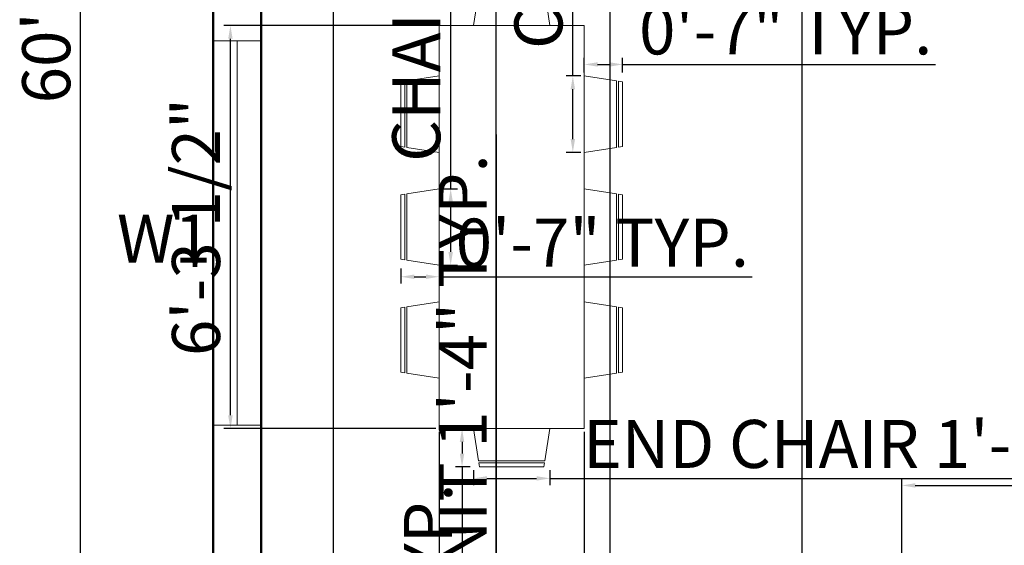
# Model space of a CAD drawing. Units: inches. Extents: x 3587 to 4539, y 1613 to 2440.
# Tile 3 of 8: x 3608 to 3793, y 1928 to 2027. Entities that reach past the tile are written whole.
import ezdxf

# ---------------------------------------------------------------- set-up
doc = ezdxf.new("R2010")
doc.units = ezdxf.units.IN
for name, color, linetype, lineweight in [('A-ANNO-DIMS', 2, 'Continuous', 18), ('A-ANNO-TEXT', 7, 'Continuous', 18), ('A-FURN', 8, 'Continuous', 18), ('A-GLAZ', 4, 'Continuous', 20), ('A-WALL', 7, 'Continuous', 50)]:
    doc.layers.add(name, color=color, linetype=linetype, lineweight=lineweight)
doc.styles.get("Standard").update_dxf_attribs({"font": 'arial.ttf'})
doc.dimstyles.new('ISO-25', dxfattribs={"dimtxt": 9, "dimasz": 2.5, "dimexe": 1.25, "dimexo": 0.625, "dimtad": 1, "dimlunit": 3, "dimtxsty": 'Standard', "dimcen": 2.5, "dimadec": 0, "dimazin": 0, "dimtfac": 1, "dimtmove": 0, "dimatfit": 3, "dimfxl": 1, "dimarcsym": 0})

# ---------------------------------------------------------------- blocks, each defined once
blk = doc.blocks.new('*D14')
at = {"layer": 'A-ANNO-DIMS', "color": 0, "lineweight": -2, "transparency": 16777216}
for p, q in [((3643.9, 2372.93), (3618.39, 2372.93)), ((3619.64, 2370.43), (3619.64, 1655.43)), ((3643.9, 1652.93), (3618.39, 1652.93))]:
    blk.add_line(p, q, dxfattribs=at)
at = {"layer": 'A-ANNO-DIMS', "color": 0, "transparency": 16777216}
for points in [[(3619.22, 2370.43), (3620.05, 2370.43), (3619.64, 2372.93)], [(3619.22, 1655.43), (3620.05, 1655.43), (3619.64, 1652.93)]]:
    blk.add_solid(points, dxfattribs=at)
at = {"layer": 'Defpoints', "color": 0, "transparency": 16777216}
for p in [(3644.52, 2372.93), (3619.64, 1652.93), (3644.52, 1652.93)]:
    blk.add_point(p, dxfattribs=at)
at = {"layer": 'A-ANNO-DIMS', "color": 0, "transparency": 16777216, "insert": (3614.42, 2019.45), "char_height": 9, "attachment_point": 5, "rotation": 90}
blk.add_mtext("60'", dxfattribs=at)
blk = doc.blocks.new('*D27')
at = {"layer": 'A-ANNO-DIMS', "color": 0, "lineweight": -2, "transparency": 16777216}
for p, q in [((3773.52, 1812.56), (3773.52, 1940.63)), ((3995.52, 1812.56), (3995.52, 1940.63)), ((3776.02, 1939.38), (3993.02, 1939.38))]:
    blk.add_line(p, q, dxfattribs=at)
at = {"layer": 'A-ANNO-DIMS', "color": 0, "transparency": 16777216}
for points in [[(3776.02, 1939.8), (3776.02, 1938.96), (3773.52, 1939.38)], [(3993.02, 1939.8), (3993.02, 1938.96), (3995.52, 1939.38)]]:
    blk.add_solid(points, dxfattribs=at)
at = {"layer": 'Defpoints', "color": 0, "transparency": 16777216}
for p in [(3995.52, 1939.38), (3773.52, 1811.93), (3995.52, 1811.93)]:
    blk.add_point(p, dxfattribs=at)
at = {"layer": 'A-ANNO-DIMS', "color": 0, "transparency": 16777216, "insert": (3884.52, 1944.6), "char_height": 9, "attachment_point": 5}
blk.add_mtext('18\'-6"', dxfattribs=at)
blk = doc.blocks.new('DINING-CHAIR-SIDE-R')
for p, q in [((6.04, 13.38), (0, 14.32)), ((6.04, 13.37), (6.04, 0.94)), ((7.17, 13.2), (6.42, 13.32)), ((6.42, 1), (6.42, 13.31)), ((7.17, 13.2), (7.17, 1.12)), ((0, 0), (6.04, 0.94)), ((6.42, 1), (7.17, 1.12))]:
    blk.add_line(p, q)
blk = doc.blocks.new('DINING-CHAIR-SIDE-L')
for p, q in [((0, 13.2), (0.75, 13.32)), ((0, 13.2), (0, 1.12)), ((0.75, 1), (0.75, 13.31)), ((1.13, 13.38), (7.17, 14.32)), ((1.13, 13.37), (1.13, 0.94)), ((0.75, 1), (0, 1.12)), ((7.17, 0), (1.13, 0.94))]:
    blk.add_line(p, q)
blk = doc.blocks.new('DINING-CHAIR-END')
for p, q in [((0, 0), (0.94, 6.04)), ((13.37, 6.04), (0.94, 6.04)), ((1, 6.42), (1.12, 7.17)), ((1, 6.42), (13.32, 6.42)), ((13.2, 7.17), (1.12, 7.17)), ((13.2, 7.17), (13.32, 6.42)), ((13.38, 6.04), (14.32, 0))]:
    blk.add_line(p, q)
blk = doc.blocks.new('*D70')
at = {"layer": 'A-ANNO-DIMS', "color": 0, "lineweight": -2, "transparency": 16777216}
for p, q in [((3697.61, 1857.46), (3697.61, 2005.08)), ((3695.87, 1857.46), (3698.86, 1857.46)), ((3697.61, 1844.2), (3697.61, 1854.96)), ((3695.87, 1841.7), (3698.86, 1841.7))]:
    blk.add_line(p, q, dxfattribs=at)
at = {"layer": 'A-ANNO-DIMS', "color": 0, "transparency": 16777216}
for points in [[(3697.19, 1854.96), (3698.02, 1854.96), (3697.61, 1857.46)], [(3697.19, 1844.2), (3698.02, 1844.2), (3697.61, 1841.7)]]:
    blk.add_solid(points, dxfattribs=at)
at = {"layer": 'Defpoints', "color": 0, "transparency": 16777216}
for p in [(3695.24, 1857.46), (3697.61, 1857.46), (3695.24, 1841.7)]:
    blk.add_point(p, dxfattribs=at)
at = {"layer": 'A-ANNO-DIMS', "color": 0, "transparency": 16777216, "insert": (3692.39, 1932.52), "char_height": 9, "attachment_point": 5, "rotation": 90}
blk.add_mtext('BURNER UNIT 1\'-4" TYP.', dxfattribs=at)
blk = doc.blocks.new('*D74')
at = {"layer": 'A-ANNO-DIMS', "color": 0, "lineweight": -2, "transparency": 16777216}
for p, q in [((3711.88, 2016.07), (3711.88, 2138.15)), ((3713.4, 2016.07), (3710.63, 2016.07)), ((3711.88, 2004.25), (3711.88, 2013.57)), ((3713.4, 2001.75), (3710.63, 2001.75))]:
    blk.add_line(p, q, dxfattribs=at)
at = {"layer": 'A-ANNO-DIMS', "color": 0, "transparency": 16777216}
for points in [[(3711.46, 2013.57), (3712.29, 2013.57), (3711.88, 2016.07)], [(3711.46, 2004.25), (3712.29, 2004.25), (3711.88, 2001.75)]]:
    blk.add_solid(points, dxfattribs=at)
at = {"layer": 'Defpoints', "color": 0, "transparency": 16777216}
for p in [(3711.88, 2016.07), (3714.02, 2016.07), (3714.02, 2001.75)]:
    blk.add_point(p, dxfattribs=at)
at = {"layer": 'A-ANNO-DIMS', "color": 0, "transparency": 16777216, "insert": (3706.6, 2078.36), "char_height": 9, "attachment_point": 5, "rotation": 90}
blk.add_mtext('CHAIR 1\'-2 1/2" TYP.', dxfattribs=at)
blk = doc.blocks.new('*D75')
at = {"layer": 'A-ANNO-DIMS', "color": 0, "lineweight": -2, "transparency": 16777216}
for p, q in [((3714.02, 2016.69), (3714.02, 2019.46)), ((3721.2, 2016.69), (3721.2, 2019.46)), ((3716.52, 2018.21), (3718.7, 2018.21)), ((3721.2, 2018.21), (3779.81, 2018.21))]:
    blk.add_line(p, q, dxfattribs=at)
at = {"layer": 'A-ANNO-DIMS', "color": 0, "transparency": 16777216}
for points in [[(3716.52, 2018.63), (3716.52, 2017.8), (3714.02, 2018.21)], [(3718.7, 2018.63), (3718.7, 2017.8), (3721.2, 2018.21)]]:
    blk.add_solid(points, dxfattribs=at)
at = {"layer": 'Defpoints', "color": 0, "transparency": 16777216}
for p in [(3721.2, 2018.21), (3714.02, 2016.07), (3721.2, 2016.07)]:
    blk.add_point(p, dxfattribs=at)
at = {"layer": 'A-ANNO-DIMS', "color": 0, "transparency": 16777216, "insert": (3751.75, 2023.43), "char_height": 9, "attachment_point": 5}
blk.add_mtext('0\'-7" TYP.', dxfattribs=at)
blk = doc.blocks.new('*D76')
at = {"layer": 'A-ANNO-DIMS', "color": 0, "lineweight": -2, "transparency": 16777216}
for p, q in [((3689, 1994.93), (3689, 2117.02)), ((3687.48, 1994.93), (3690.25, 1994.93)), ((3689, 1983.11), (3689, 1992.43)), ((3687.48, 1980.61), (3690.25, 1980.61))]:
    blk.add_line(p, q, dxfattribs=at)
at = {"layer": 'A-ANNO-DIMS', "color": 0, "transparency": 16777216}
for points in [[(3688.58, 1992.43), (3689.42, 1992.43), (3689, 1994.93)], [(3688.58, 1983.11), (3689.42, 1983.11), (3689, 1980.61)]]:
    blk.add_solid(points, dxfattribs=at)
at = {"layer": 'Defpoints', "color": 0, "transparency": 16777216}
for p in [(3686.85, 1994.93), (3689, 1994.93), (3686.85, 1980.61)]:
    blk.add_point(p, dxfattribs=at)
at = {"layer": 'A-ANNO-DIMS', "color": 0, "transparency": 16777216, "insert": (3683.72, 2057.22), "char_height": 9, "attachment_point": 5, "rotation": 90}
blk.add_mtext('CHAIR 1\'-2 1/2" TYP.', dxfattribs=at)
blk = doc.blocks.new('*D77')
at = {"layer": 'A-ANNO-DIMS', "color": 0, "lineweight": -2, "transparency": 16777216}
for p, q in [((3679.68, 1979.98), (3679.68, 1977.21)), ((3686.85, 1979.98), (3686.85, 1977.21)), ((3682.18, 1978.46), (3684.35, 1978.46)), ((3686.85, 1978.46), (3745.46, 1978.46))]:
    blk.add_line(p, q, dxfattribs=at)
at = {"layer": 'A-ANNO-DIMS', "color": 0, "transparency": 16777216}
for points in [[(3682.18, 1978.88), (3682.18, 1978.04), (3679.68, 1978.46)], [(3684.35, 1978.88), (3684.35, 1978.04), (3686.85, 1978.46)]]:
    blk.add_solid(points, dxfattribs=at)
at = {"layer": 'Defpoints', "color": 0, "transparency": 16777216}
for p in [(3679.68, 1980.61), (3686.85, 1980.61), (3686.85, 1978.46)]:
    blk.add_point(p, dxfattribs=at)
at = {"layer": 'A-ANNO-DIMS', "color": 0, "transparency": 16777216, "insert": (3717.41, 1983.68), "char_height": 9, "attachment_point": 5}
blk.add_mtext('0\'-7" TYP.', dxfattribs=at)
blk = doc.blocks.new('*D78')
at = {"layer": 'A-ANNO-DIMS', "color": 0, "lineweight": -2, "transparency": 16777216}
for p, q in [((3693.28, 1942.22), (3693.28, 1939.45)), ((3707.6, 1942.22), (3707.6, 1939.45)), ((3695.78, 1940.7), (3705.1, 1940.7)), ((3707.6, 1940.7), (3859.36, 1940.7))]:
    blk.add_line(p, q, dxfattribs=at)
at = {"layer": 'A-ANNO-DIMS', "color": 0, "transparency": 16777216}
for points in [[(3695.78, 1941.11), (3695.78, 1940.28), (3693.28, 1940.7)], [(3705.1, 1941.11), (3705.1, 1940.28), (3707.6, 1940.7)]]:
    blk.add_solid(points, dxfattribs=at)
at = {"layer": 'Defpoints', "color": 0, "transparency": 16777216}
for p in [(3693.28, 1942.85), (3707.6, 1942.85), (3707.6, 1940.7)]:
    blk.add_point(p, dxfattribs=at)
at = {"layer": 'A-ANNO-DIMS', "color": 0, "transparency": 16777216, "insert": (3784.73, 1945.98), "char_height": 9, "attachment_point": 5}
blk.add_mtext('END CHAIR 1\'-2 1/2" TYP.', dxfattribs=at)
blk = doc.blocks.new('*D79')
at = {"layer": 'A-ANNO-DIMS', "color": 0, "lineweight": -2, "transparency": 16777216}
for p, q in [((3692.65, 1950.02), (3689.88, 1950.02)), ((3691.13, 1947.52), (3691.13, 1945.35)), ((3692.65, 1942.85), (3689.88, 1942.85)), ((3691.13, 1942.85), (3691.13, 1884.24))]:
    blk.add_line(p, q, dxfattribs=at)
at = {"layer": 'A-ANNO-DIMS', "color": 0, "transparency": 16777216}
for points in [[(3690.71, 1947.52), (3691.55, 1947.52), (3691.13, 1950.02)], [(3690.71, 1945.35), (3691.55, 1945.35), (3691.13, 1942.85)]]:
    blk.add_solid(points, dxfattribs=at)
at = {"layer": 'Defpoints', "color": 0, "transparency": 16777216}
for p in [(3693.28, 1950.02), (3691.13, 1942.85), (3693.28, 1942.85)]:
    blk.add_point(p, dxfattribs=at)
at = {"layer": 'A-ANNO-DIMS', "color": 0, "transparency": 16777216, "insert": (3685.91, 1912.29), "char_height": 9, "attachment_point": 5, "rotation": 90}
blk.add_mtext('0\'-7" TYP.', dxfattribs=at)
blk = doc.blocks.new('*D84')
at = {"layer": 'A-ANNO-DIMS', "color": 0, "lineweight": -2, "transparency": 16777216}
for p, q in [((3686.23, 2025.51), (3646.5, 2025.51)), ((3647.75, 1952.52), (3647.75, 2023.01)), ((3686.23, 1950.02), (3646.5, 1950.02))]:
    blk.add_line(p, q, dxfattribs=at)
at = {"layer": 'A-ANNO-DIMS', "color": 0, "transparency": 16777216}
for points in [[(3647.33, 2023.01), (3648.17, 2023.01), (3647.75, 2025.51)], [(3647.33, 1952.52), (3648.17, 1952.52), (3647.75, 1950.02)]]:
    blk.add_solid(points, dxfattribs=at)
at = {"layer": 'Defpoints', "color": 0, "transparency": 16777216}
for p in [(3647.75, 2025.51), (3686.85, 2025.51), (3686.85, 1950.02)]:
    blk.add_point(p, dxfattribs=at)
at = {"layer": 'A-ANNO-DIMS', "color": 0, "transparency": 16777216, "insert": (3642.47, 1987.77), "char_height": 9, "attachment_point": 5, "rotation": 90}
blk.add_mtext('6\'-3 1/2"', dxfattribs=at)
blk = doc.blocks.new('*D85')
at = {"layer": 'A-ANNO-DIMS', "color": 0, "lineweight": -2, "transparency": 16777216}
for p, q in [((3686.85, 1949.39), (3686.85, 1909.67)), ((3714.03, 1949.39), (3714.03, 1909.67)), ((3711.53, 1910.92), (3689.35, 1910.92))]:
    blk.add_line(p, q, dxfattribs=at)
at = {"layer": 'A-ANNO-DIMS', "color": 0, "transparency": 16777216}
for points in [[(3689.35, 1911.33), (3689.35, 1910.5), (3686.85, 1910.92)], [(3711.53, 1911.33), (3711.53, 1910.5), (3714.03, 1910.92)]]:
    blk.add_solid(points, dxfattribs=at)
at = {"layer": 'Defpoints', "color": 0, "transparency": 16777216}
for p in [(3686.85, 1950.02), (3714.03, 1950.02), (3686.85, 1910.92)]:
    blk.add_point(p, dxfattribs=at)
at = {"layer": 'A-ANNO-DIMS', "color": 0, "transparency": 16777216, "insert": (3700.44, 1916.14), "char_height": 9, "attachment_point": 5}
blk.add_mtext('2\'-3"', dxfattribs=at)
blk = doc.blocks.new('*D96')
at = {"layer": 'A-ANNO-DIMS', "color": 0, "lineweight": -2, "transparency": 16777216}
for p, q in [((3667.04, 1858.35), (3667.04, 2413.28)), ((3669.54, 2412.03), (3695.05, 2412.03)), ((3697.55, 1858.35), (3697.55, 2413.28)), ((3697.55, 2412.03), (3746.35, 2412.03))]:
    blk.add_line(p, q, dxfattribs=at)
at = {"layer": 'A-ANNO-DIMS', "color": 0, "transparency": 16777216}
for points in [[(3669.54, 2412.45), (3669.54, 2411.62), (3667.04, 2412.03)], [(3695.05, 2412.45), (3695.05, 2411.62), (3697.55, 2412.03)]]:
    blk.add_solid(points, dxfattribs=at)
at = {"layer": 'Defpoints', "color": 0, "transparency": 16777216}
for p in [(3697.55, 2412.03), (3667.04, 1857.73), (3697.55, 1857.73)]:
    blk.add_point(p, dxfattribs=at)
at = {"layer": 'A-ANNO-DIMS', "color": 0, "transparency": 16777216, "insert": (3723.2, 2417.31), "char_height": 9, "attachment_point": 5}
blk.add_mtext('2\'-6 1/2"', dxfattribs=at)
blk = doc.blocks.new('*D98')
at = {"layer": 'A-ANNO-DIMS', "color": 0, "lineweight": -2, "transparency": 16777216}
for p, q in [((3718.85, 1857.52), (3718.85, 2413.28)), ((3721.35, 2412.03), (3752.35, 2412.03)), ((3754.85, 1857.52), (3754.85, 2413.28))]:
    blk.add_line(p, q, dxfattribs=at)
at = {"layer": 'A-ANNO-DIMS', "color": 0, "transparency": 16777216}
for points in [[(3721.35, 2412.45), (3721.35, 2411.62), (3718.85, 2412.03)], [(3752.35, 2412.45), (3752.35, 2411.62), (3754.85, 2412.03)]]:
    blk.add_solid(points, dxfattribs=at)
at = {"layer": 'Defpoints', "color": 0, "transparency": 16777216}
for p in [(3754.85, 2412.03), (3718.85, 1856.9), (3754.85, 1856.9)]:
    blk.add_point(p, dxfattribs=at)
at = {"layer": 'A-ANNO-DIMS', "color": 0, "transparency": 16777216, "insert": (3736.85, 2417.26), "char_height": 9, "attachment_point": 5}
blk.add_mtext('3\'-0"', dxfattribs=at)

msp = doc.modelspace()

# ---------------------------------------------------------------- linework, layer by layer
at = {"layer": 'A-FURN'}
for p, q in [((3686.85, 2025.513), (3686.85, 1950.017)), ((3714.027, 2025.513), (3686.85, 2025.513)), ((3714.027, 1950.017), (3714.027, 2025.513)), ((3714.027, 1950.017), (3686.85, 1950.017))]:
    msp.add_line(p, q, dxfattribs=at)
at = {"layer": 'A-GLAZ'}
for p, q in [((3644.523, 2022.643), (3653.523, 2022.643)), ((3649.023, 2022.643), (3649.023, 1950.643)), ((3644.523, 1950.643), (3653.523, 1950.643))]:
    msp.add_line(p, q, dxfattribs=at)
at = {"layer": 'A-WALL'}
for p, q in [((3644.523, 2372.933), (3644.523, 1652.933)), ((3653.523, 2051.933), (3653.523, 1835.933))]:
    msp.add_line(p, q, dxfattribs=at)

# ---------------------------------------------------------------- block references
at = {"layer": 'A-FURN'}
for name, p in [('DINING-CHAIR-END', (3693.278, 2025.512)), ('DINING-CHAIR-SIDE-L', (3679.679, 2001.746)), ('DINING-CHAIR-SIDE-R', (3714.025, 2001.746)), ('DINING-CHAIR-SIDE-L', (3679.679, 1980.609)), ('DINING-CHAIR-SIDE-R', (3714.025, 1980.609))]:
    msp.add_blockref(name, p, dxfattribs=at)
at = {"layer": 'A-FURN', "extrusion": (0, 0, -1), "zscale": -1, "rotation": 180}
for name, p in [('DINING-CHAIR-SIDE-L', (-3679.679, 1973.785)), ('DINING-CHAIR-SIDE-R', (-3714.025, 1973.785)), ('DINING-CHAIR-END', (-3693.278, 1950.019))]:
    msp.add_blockref(name, p, dxfattribs=at)

# ---------------------------------------------------------------- texts
at = {"layer": 'A-ANNO-TEXT', "insert": (3626.499, 1990.101), "char_height": 9, "attachment_point": 1}
msp.add_mtext_dynamic_manual_height_columns('W1', width=34.45655, gutter_width=12.5, heights=[0], dxfattribs=at)

# ---------------------------------------------------------------- dimensions: what is measured, and where the dimension line sits
at = {"layer": 'A-ANNO-DIMS'}
for base, p1, p2, override, picture, middle in [((3697.551, 2412.033), (3667.042, 1857.729), (3697.551, 1857.729), {"dimdec": 1, "dimlfac": 1, "dimrnd": 0, "dimzin": 1, "dimdsep": 46, "dimlunit": 4, "dimfrac": 2}, '*D96', (3723.2, 2417.312)), ((3754.854, 2412.033), (3718.854, 1856.898), (3754.854, 1856.898), {"dimdec": 1, "dimlfac": 1, "dimrnd": 0, "dimzin": 1, "dimdsep": 46, "dimlunit": 4, "dimfrac": 2}, '*D98', (3736.854, 2417.256)), ((3995.523, 1939.381), (3773.523, 1811.933), (3995.523, 1811.933), {"dimclrd": 0, "dimclre": 0, "dimclrt": 0}, '*D27', (3884.523, 1944.601))]:
    dim = msp.add_linear_dim(base=base, p1=p1, p2=p2, dimstyle='ISO-25', override=override, dxfattribs=at)
    dim.commit()
    dim.dimension.update_dxf_attribs({"geometry": picture, "text_midpoint": middle})
dim = msp.add_linear_dim(base=(3619.637, 1652.933), p1=(3644.523, 2372.933), p2=(3644.523, 1652.933), angle=90, dimstyle='ISO-25', override={"dimclrd": 0, "dimclre": 0, "dimclrt": 0}, dxfattribs=at)
dim.commit()
dim.dimension.update_dxf_attribs({"geometry": '*D14', "text_midpoint": (3619.637, 2019.453), "dimtype": 160})
for base, p1, p2, angle, text, picture, middle in [((3711.877, 2016.066), (3714.025, 2001.746), (3714.025, 2016.066), 90, 'CHAIR <> TYP.', '*D74', (3706.598, 2078.36)), ((3689, 1994.929), (3686.852, 1980.609), (3686.852, 1994.929), 90, 'CHAIR <> TYP.', '*D76', (3683.722, 2057.223)), ((3697.608, 1857.458), (3695.244, 1841.696), (3695.244, 1857.458), 90, 'BURNER UNIT <> TYP.', '*D70', (3692.388, 1932.518)), ((3691.13, 1942.846), (3693.278, 1950.019), (3693.278, 1942.846), 270, '<> TYP.', '*D79', (3685.91, 1912.291))]:
    dim = msp.add_linear_dim(base=base, p1=p1, p2=p2, angle=angle, text=text, dimstyle='ISO-25', override={"dimdec": 1, "dimlfac": 1, "dimrnd": 0, "dimzin": 1, "dimdsep": 46, "dimlunit": 4, "dimfrac": 2}, dxfattribs=at)
    dim.commit()
    dim.dimension.update_dxf_attribs({"geometry": picture, "text_midpoint": middle})
for base, p1, p2, text, picture, middle in [((3721.198, 2018.214), (3714.025, 2016.066), (3721.198, 2016.066), '<> TYP.', '*D75', (3751.753, 2023.434)), ((3686.852, 1978.461), (3679.679, 1980.609), (3686.852, 1980.609), '<> TYP.', '*D77', (3717.407, 1983.681)), ((3707.598, 1940.698), (3693.278, 1942.846), (3707.598, 1942.846), 'END CHAIR <> TYP.', '*D78', (3784.728, 1945.976))]:
    dim = msp.add_linear_dim(base=base, p1=p1, p2=p2, text=text, dimstyle='ISO-25', override={"dimdec": 1, "dimlfac": 1, "dimrnd": 0, "dimzin": 1, "dimdsep": 46, "dimlunit": 4, "dimfrac": 2}, dxfattribs=at)
    dim.commit()
    dim.dimension.update_dxf_attribs({"geometry": picture, "text_midpoint": middle})
for base, p1, p2, angle, picture, middle in [((3647.75, 2025.513), (3686.85, 1950.017), (3686.85, 2025.513), 90, '*D84', (3642.469, 1987.765)), ((3686.85, 1910.917), (3714.027, 1950.017), (3686.85, 1950.017), 180, '*D85', (3700.439, 1916.14))]:
    dim = msp.add_linear_dim(base=base, p1=p1, p2=p2, angle=angle, dimstyle='ISO-25', override={"dimdec": 1, "dimlfac": 1, "dimrnd": 0, "dimzin": 1, "dimdsep": 46, "dimlunit": 4, "dimfrac": 2}, dxfattribs=at)
    dim.commit()
    dim.dimension.update_dxf_attribs({"geometry": picture, "text_midpoint": middle})

doc.saveas('drawing.dxf')
